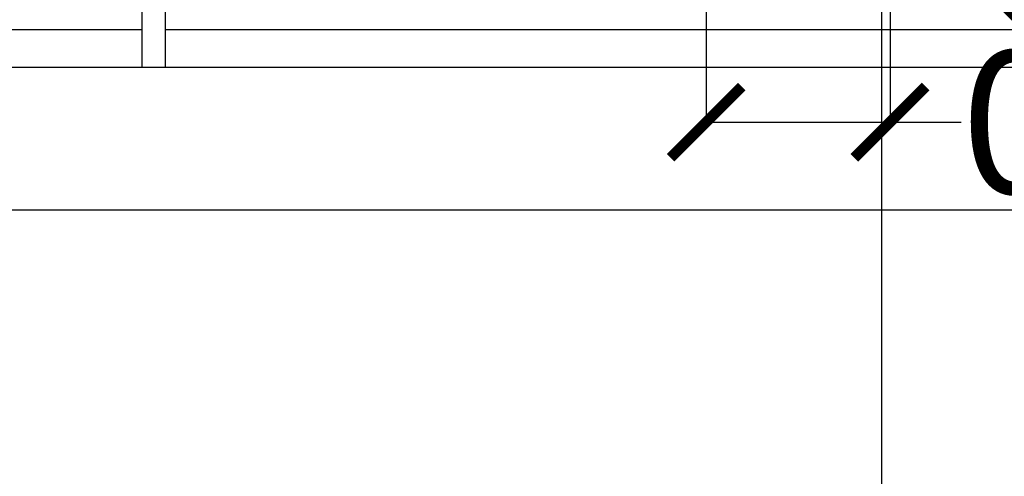
# Model space of a CAD drawing. Units: inches. Extents: x 2278 to 7495, y -71 to 1198.
# Tile 22 of 44: x 5060 to 5101, y 107 to 126. Entities that reach past the tile are written whole.
import ezdxf

# ---------------------------------------------------------------- set-up
doc = ezdxf.new("R2010")
doc.units = ezdxf.units.IN
doc.header["$MEASUREMENT"] = 0
doc.layers.add('A-ANNO-DIMS', color=2, linetype='Continuous', lineweight=18)
doc.layers.add('A-ELEV', color=7, linetype='Continuous', lineweight=25)
doc.styles.get("Standard").update_dxf_attribs({"font": 'arial.ttf'})
doc.dimstyles.get("Standard").update_dxf_attribs({"dimtxt": 6, "dimasz": 3, "dimexe": 0.18, "dimexo": 0.0625, "dimgap": 0.09, "dimtad": 0, "dimtih": 1, "dimtoh": 1, "dimdec": 0, "dimzin": 0, "dimdsep": 46, "dimlunit": 3, "dimtxsty": 'Standard', "dimblk": 'ARCHTICK', "dimcen": 0.09, "dimadec": 0, "dimazin": 0, "dimtfac": 1, "dimtdec": 0, "dimtofl": 0, "dimtmove": 0, "dimatfit": 3, "dimfxl": 1, "dimtolj": 1, "dimtzin": 0, "dimarcsym": 0})

# ---------------------------------------------------------------- blocks, each defined once
blk = doc.blocks.new('_ArchTick')
at = {"color": 0, "linetype": 'ByBlock', "const_width": 0.15}
blk.add_lwpolyline([(-0.5, -0.5), (0.5, 0.5)], dxfattribs=at)
blk = doc.blocks.new('*D59')
at = {"layer": 'A-ANNO-DIMS', "color": 0, "lineweight": -2, "transparency": 16777216}
for p, q in [((5096.589, 159.183), (5101.564, 159.183)), ((5101.384, 159.183), (5101.384, 146.185)), ((5101.384, 126.799), (5101.384, 139.796)), ((5096.589, 126.799), (5101.564, 126.799))]:
    blk.add_line(p, q, dxfattribs=at)
at = {"layer": 'Defpoints', "color": 0, "transparency": 16777216}
for p in [(5096.527, 159.183), (5101.384, 159.183), (5096.527, 126.799)]:
    blk.add_point(p, dxfattribs=at)
at = {"layer": 'A-ANNO-DIMS', "color": 0, "lineweight": -2, "transparency": 16777216, "xscale": 3, "yscale": 3, "zscale": 3}
for p, rotation in [((5101.384, 159.183), 90), ((5101.384, 126.799), 270)]:
    blk.add_blockref('_ArchTick', p, dxfattribs=dict(at, rotation=rotation))
at = {"layer": 'A-ANNO-DIMS', "color": 0, "transparency": 16777216, "insert": (5101.384, 142.991), "char_height": 6, "attachment_point": 5}
blk.add_mtext('\\A1;ORNATE BALUSTER 2\'-8 1/2" TYP.', dxfattribs=at)
blk = doc.blocks.new('*D60')
at = {"layer": 'A-ANNO-DIMS', "color": 0, "lineweight": -2, "transparency": 16777216}
for p, q in [((5088.787, 126.736), (5088.787, 121.761)), ((5096.527, 126.736), (5096.527, 121.761)), ((5088.787, 121.941), (5096.527, 121.941)), ((5096.527, 121.941), (5099.527, 121.941))]:
    blk.add_line(p, q, dxfattribs=at)
at = {"layer": 'Defpoints', "color": 0, "transparency": 16777216}
for p in [(5088.787, 126.799), (5096.527, 126.799), (5096.527, 121.941)]:
    blk.add_point(p, dxfattribs=at)
at = {"layer": 'A-ANNO-DIMS', "color": 0, "lineweight": -2, "transparency": 16777216, "xscale": 3, "yscale": 3, "zscale": 3, "rotation": 180}
blk.add_blockref('_ArchTick', (5088.787, 121.941), dxfattribs=at)
at = {"layer": 'A-ANNO-DIMS', "color": 0, "lineweight": -2, "transparency": 16777216, "xscale": 3, "yscale": 3, "zscale": 3}
blk.add_blockref('_ArchTick', (5096.527, 121.941), dxfattribs=at)
at = {"layer": 'A-ANNO-DIMS', "color": 0, "transparency": 16777216, "insert": (5124.894, 121.941), "char_height": 6, "attachment_point": 5}
blk.add_mtext('\\A1;0\'-7 1/2" TYP.', dxfattribs=at)
blk = doc.blocks.new('*D123')
at = {"layer": 'A-ANNO-DIMS', "color": 0, "lineweight": -2, "transparency": 16777216}
for p, q in [((4736.95, 340.157), (4736.95, -23.427)), ((5145.676, -1.81), (5145.676, -23.427)), ((4736.95, -23.247), (4923.929, -23.247)), ((5145.676, -23.247), (4958.697, -23.247))]:
    blk.add_line(p, q, dxfattribs=at)
at = {"layer": 'Defpoints', "color": 0, "transparency": 16777216}
for p in [(4736.95, 340.219), (5145.676, -1.747), (5145.676, -23.247)]:
    blk.add_point(p, dxfattribs=at)
at = {"layer": 'A-ANNO-DIMS', "color": 0, "lineweight": -2, "transparency": 16777216, "xscale": 3, "yscale": 3, "zscale": 3, "rotation": 180}
blk.add_blockref('_ArchTick', (4736.95, -23.247), dxfattribs=at)
at = {"layer": 'A-ANNO-DIMS', "color": 0, "lineweight": -2, "transparency": 16777216, "xscale": 3, "yscale": 3, "zscale": 3}
blk.add_blockref('_ArchTick', (5145.676, -23.247), dxfattribs=at)
at = {"layer": 'A-ANNO-DIMS', "color": 0, "transparency": 16777216, "insert": (4941.313, -23.247), "char_height": 6, "attachment_point": 5}
blk.add_mtext('\\A1;34\'-0 1/2"', dxfattribs=at)
blk = doc.blocks.new('*D130')
at = {"layer": 'A-ANNO-DIMS', "color": 0, "lineweight": -2, "transparency": 16777216}
for p, q in [((5016.176, 99.315), (5016.176, 361.899)), ((5016.176, 361.719), (5048.095, 361.719)), ((5096.176, 361.719), (5064.257, 361.719)), ((5096.176, 99.315), (5096.176, 361.899))]:
    blk.add_line(p, q, dxfattribs=at)
at = {"layer": 'Defpoints', "color": 0, "transparency": 16777216}
for p in [(5096.176, 361.719), (5016.176, 99.253), (5096.176, 99.253)]:
    blk.add_point(p, dxfattribs=at)
at = {"layer": 'A-ANNO-DIMS', "color": 0, "lineweight": -2, "transparency": 16777216, "xscale": 3, "yscale": 3, "zscale": 3, "rotation": 180}
blk.add_blockref('_ArchTick', (5016.176, 361.719), dxfattribs=at)
at = {"layer": 'A-ANNO-DIMS', "color": 0, "lineweight": -2, "transparency": 16777216, "xscale": 3, "yscale": 3, "zscale": 3}
blk.add_blockref('_ArchTick', (5096.176, 361.719), dxfattribs=at)
at = {"layer": 'A-ANNO-DIMS', "color": 0, "transparency": 16777216, "insert": (5056.176, 361.719), "char_height": 6, "attachment_point": 5}
blk.add_mtext('\\A1;6\'-8"', dxfattribs=at)
blk = doc.blocks.new('*D131')
at = {"layer": 'A-ANNO-DIMS', "color": 0, "lineweight": -2, "transparency": 16777216}
for p, q in [((5096.176, 99.315), (5096.176, 361.899)), ((5096.176, 361.719), (5105.75, 361.719)), ((5145.676, 361.719), (5136.102, 361.719)), ((5145.676, 118.315), (5145.676, 361.899))]:
    blk.add_line(p, q, dxfattribs=at)
at = {"layer": 'Defpoints', "color": 0, "transparency": 16777216}
for p in [(5145.676, 361.719), (5145.676, 118.253), (5096.176, 99.253)]:
    blk.add_point(p, dxfattribs=at)
at = {"layer": 'A-ANNO-DIMS', "color": 0, "lineweight": -2, "transparency": 16777216, "xscale": 3, "yscale": 3, "zscale": 3, "rotation": 180}
blk.add_blockref('_ArchTick', (5096.176, 361.719), dxfattribs=at)
at = {"layer": 'A-ANNO-DIMS', "color": 0, "lineweight": -2, "transparency": 16777216, "xscale": 3, "yscale": 3, "zscale": 3}
blk.add_blockref('_ArchTick', (5145.676, 361.719), dxfattribs=at)
at = {"layer": 'A-ANNO-DIMS', "color": 0, "transparency": 16777216, "insert": (5120.926, 361.719), "char_height": 6, "attachment_point": 5}
blk.add_mtext('\\A1;4\'-1 1/2"', dxfattribs=at)
blk = doc.blocks.new('*D138')
at = {"layer": 'A-ANNO-DIMS', "color": 0, "lineweight": -2, "transparency": 16777216}
for p, q in [((5145.739, 118.253), (5167.754, 118.253)), ((5167.574, 118.253), (5167.574, 111.855)), ((5167.574, 99.253), (5167.574, 105.651)), ((5096.239, 99.253), (5167.754, 99.253))]:
    blk.add_line(p, q, dxfattribs=at)
at = {"layer": 'Defpoints', "color": 0, "transparency": 16777216}
for p in [(5145.676, 118.253), (5167.574, 118.253), (5096.176, 99.253)]:
    blk.add_point(p, dxfattribs=at)
at = {"layer": 'A-ANNO-DIMS', "color": 0, "lineweight": -2, "transparency": 16777216, "xscale": 3, "yscale": 3, "zscale": 3}
for p, rotation in [((5167.574, 118.253), 90), ((5167.574, 99.253), 270)]:
    blk.add_blockref('_ArchTick', p, dxfattribs=dict(at, rotation=rotation))
at = {"layer": 'A-ANNO-DIMS', "color": 0, "transparency": 16777216, "insert": (5167.574, 108.753), "char_height": 6, "attachment_point": 5}
blk.add_mtext('\\A1;1\'-7"', dxfattribs=at)
blk = doc.blocks.new('*D139')
at = {"layer": 'A-ANNO-DIMS', "color": 0, "lineweight": -2, "transparency": 16777216}
for p, q in [((5092.239, 160.253), (5167.754, 160.253)), ((5167.574, 160.253), (5167.574, 142.408)), ((5167.574, 118.253), (5167.574, 136.097)), ((5145.739, 118.253), (5167.754, 118.253))]:
    blk.add_line(p, q, dxfattribs=at)
at = {"layer": 'Defpoints', "color": 0, "transparency": 16777216}
for p in [(5092.176, 160.253), (5167.574, 160.253), (5145.676, 118.253)]:
    blk.add_point(p, dxfattribs=at)
at = {"layer": 'A-ANNO-DIMS', "color": 0, "lineweight": -2, "transparency": 16777216, "xscale": 3, "yscale": 3, "zscale": 3}
for p, rotation in [((5167.574, 160.253), 90), ((5167.574, 118.253), 270)]:
    blk.add_blockref('_ArchTick', p, dxfattribs=dict(at, rotation=rotation))
at = {"layer": 'A-ANNO-DIMS', "color": 0, "transparency": 16777216, "insert": (5167.574, 139.253), "char_height": 6, "attachment_point": 5}
blk.add_mtext('\\A1;3\'-6"', dxfattribs=at)

msp = doc.modelspace()

# ---------------------------------------------------------------- linework, layer by layer
at = {"layer": 'A-ELEV'}
for p, q in [((5065.039, 124.253), (5065.039, 139.899)), ((5066.016, 124.253), (5066.016, 139.899)), ((5065.039, 125.821), (4971.673, 125.821)), ((5145.676, 125.821), (5066.016, 125.821)), ((4874.676, 124.253), (5145.676, 124.253)), ((4874.676, 118.253), (5145.676, 118.253))]:
    msp.add_line(p, q, dxfattribs=at)

# ---------------------------------------------------------------- dimensions: what is measured, and where the dimension line sits
at = {"layer": 'A-ANNO-DIMS'}
for base, p1, p2, picture, middle in [((5145.676, 361.719), (5096.176, 99.253), (5145.676, 118.253), '*D131', (5120.926, 361.719)), ((5096.176, 361.719), (5016.176, 99.253), (5096.176, 99.253), '*D130', (5056.176, 361.719)), ((5145.676, -23.247), (4736.95, 340.219), (5145.676, -1.747), '*D123', (4941.313, -23.247))]:
    dim = msp.add_linear_dim(base=base, p1=p1, p2=p2, dimstyle='Standard', override={"dimdec": 1, "dimlfac": 1, "dimrnd": 0, "dimzin": 1, "dimdsep": 46, "dimlunit": 4, "dimfrac": 2}, dxfattribs=at)
    dim.commit()
    dim.dimension.update_dxf_attribs({"geometry": picture, "text_midpoint": middle})
dim = msp.add_linear_dim(base=(5101.384, 159.183), p1=(5096.527, 126.799), p2=(5096.527, 159.183), angle=90, text='ORNATE BALUSTER <> TYP.', dimstyle='Standard', override={"dimdec": 1, "dimrnd": 0, "dimzin": 1, "dimlunit": 4, "dimfrac": 2}, dxfattribs=at)
dim.commit()
dim.dimension.update_dxf_attribs({"geometry": '*D59', "text_midpoint": (5101.384, 142.991)})
for base, p1, p2, picture, middle in [((5167.574, 160.253), (5145.676, 118.253), (5092.176, 160.253), '*D139', (5167.574, 139.253)), ((5167.574, 118.253), (5096.176, 99.253), (5145.676, 118.253), '*D138', (5167.574, 108.753))]:
    dim = msp.add_linear_dim(base=base, p1=p1, p2=p2, angle=90, dimstyle='Standard', override={"dimdec": 1, "dimlfac": 1, "dimrnd": 0, "dimzin": 1, "dimdsep": 46, "dimlunit": 4, "dimfrac": 2}, dxfattribs=at)
    dim.commit()
    dim.dimension.update_dxf_attribs({"geometry": picture, "text_midpoint": middle})
dim = msp.add_linear_dim(base=(5096.527, 121.941), p1=(5088.787, 126.799), p2=(5096.527, 126.799), text='<> TYP.', dimstyle='Standard', override={"dimdec": 1, "dimrnd": 0, "dimzin": 1, "dimlunit": 4, "dimfrac": 2}, dxfattribs=at)
dim.commit()
dim.dimension.update_dxf_attribs({"geometry": '*D60', "text_midpoint": (5124.894, 121.941)})

doc.saveas('drawing.dxf')
